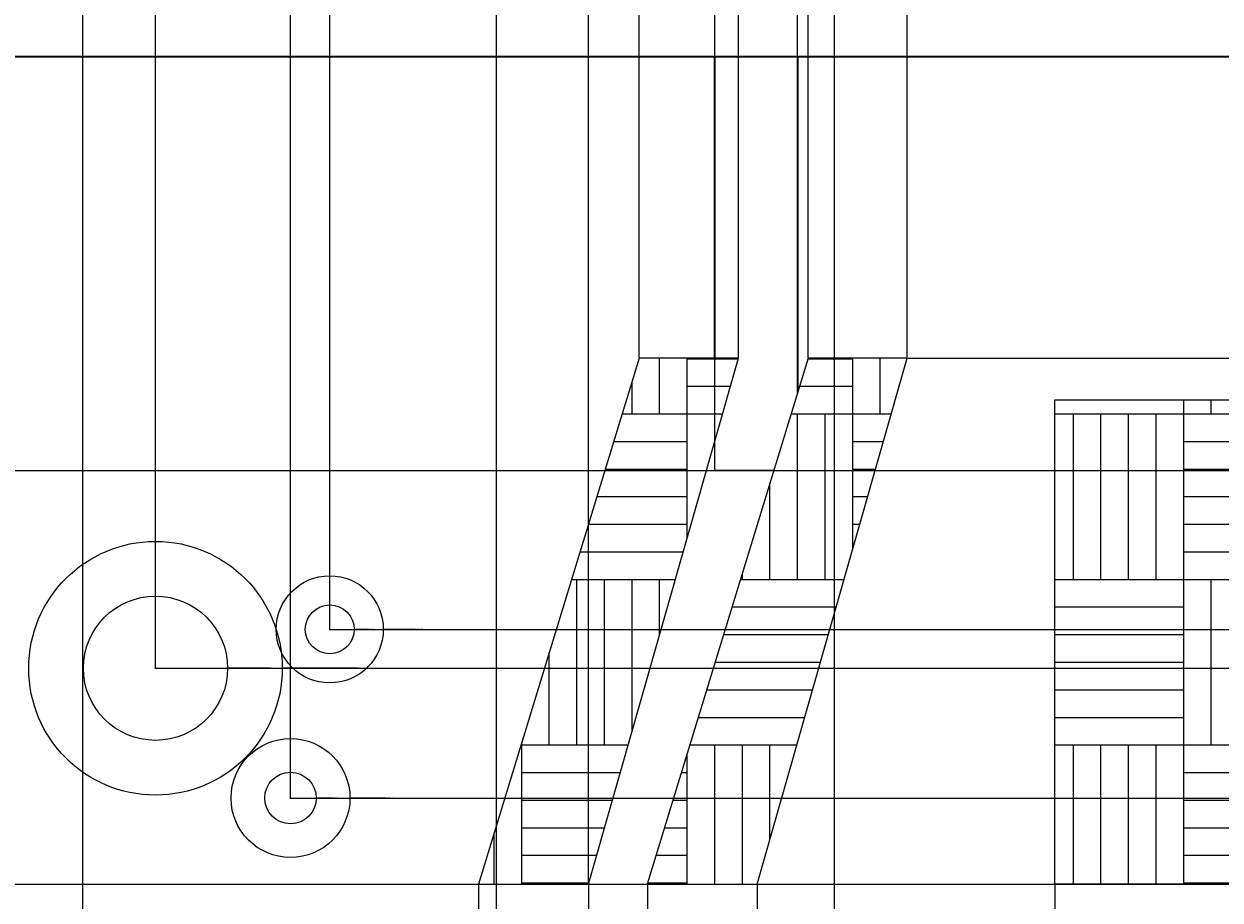
# Model space of a CAD drawing. Units: inches. Extents: x -15 to 605, y -220 to 570.
# Tile 4 of 10: x 265 to 438, y -118 to 9. Entities that reach past the tile are written whole.
import ezdxf

# ---------------------------------------------------------------- set-up
doc = ezdxf.new("R2010")
doc.units = ezdxf.units.IN
doc.header["$MEASUREMENT"] = 0
for name, color, linetype, lineweight in [('A-ANNO-DIMS', 2, 'Continuous', 18), ('A-COLS', 7, 'Continuous', 35), ('A-ELEV', 7, 'Continuous', 35), ('A-ELEV-PATT', 8, 'Continuous', 13), ('C-SITE', 3, 'Continuous', 25)]:
    doc.layers.add(name, color=color, linetype=linetype, lineweight=lineweight)
doc.styles.get("Standard").update_dxf_attribs({"font": 'arial.ttf'})
doc.dimstyles.get("Standard").update_dxf_attribs({"dimtxt": 0.18, "dimasz": 0.18, "dimexe": 0.18, "dimexo": 0.0625, "dimgap": 0.09, "dimtad": 0, "dimtih": 1, "dimtoh": 1, "dimdec": 4, "dimzin": 0, "dimdsep": 46, "dimtxsty": 'Standard', "dimcen": 0.09, "dimadec": 0, "dimazin": 0, "dimtfac": 1, "dimtdec": 4, "dimtofl": 0, "dimtmove": 0, "dimatfit": 3, "dimfxl": 1, "dimtolj": 1, "dimtzin": 0, "dimarcsym": 0})

# ---------------------------------------------------------------- blocks, each defined once
blk = doc.blocks.new('*D7')
at = {"layer": 'A-ANNO-DIMS', "color": 0, "lineweight": -2, "transparency": 16777216}
for p, q in [((23.99, 3.76), (23.99, -154.76)), ((566.72, -116.24), (566.72, -154.76)), ((24.17, -154.58), (294.96, -154.58)), ((566.54, -154.58), (295.75, -154.58))]:
    blk.add_line(p, q, dxfattribs=at)
at = {"layer": 'A-ANNO-DIMS', "color": 0, "transparency": 16777216}
for points in [[(24.17, -154.55), (24.17, -154.61), (23.99, -154.58)], [(566.54, -154.55), (566.54, -154.61), (566.72, -154.58)]]:
    blk.add_solid(points, dxfattribs=at)
at = {"layer": 'Defpoints', "color": 0, "transparency": 16777216}
for p in [(23.99, 3.82), (566.72, -116.18), (566.72, -154.58)]:
    blk.add_point(p, dxfattribs=at)
at = {"layer": 'A-ANNO-DIMS', "color": 0, "transparency": 16777216, "insert": (295.35, -154.58), "char_height": 0.18, "attachment_point": 5}
blk.add_mtext('\\A1;542.7', dxfattribs=at)
blk = doc.blocks.new('*D8')
at = {"layer": 'A-ANNO-DIMS', "color": 0, "lineweight": -2, "transparency": 16777216}
for p, q in [((23.99, 3.88), (23.99, 570.4)), ((24.17, 570.22), (263.7, 570.22)), ((503.81, 570.22), (264.28, 570.22)), ((503.99, 531.88), (503.99, 570.4))]:
    blk.add_line(p, q, dxfattribs=at)
at = {"layer": 'A-ANNO-DIMS', "color": 0, "transparency": 16777216}
for points in [[(24.17, 570.25), (24.17, 570.19), (23.99, 570.22)], [(503.81, 570.25), (503.81, 570.19), (503.99, 570.22)]]:
    blk.add_solid(points, dxfattribs=at)
at = {"layer": 'Defpoints', "color": 0, "transparency": 16777216}
for p in [(503.99, 570.22), (503.99, 531.82), (23.99, 3.82)]:
    blk.add_point(p, dxfattribs=at)
at = {"layer": 'A-ANNO-DIMS', "color": 0, "transparency": 16777216, "insert": (263.99, 570.22), "char_height": 0.18, "attachment_point": 5}
blk.add_mtext('\\A1;480', dxfattribs=at)
blk = doc.blocks.new('*D9')
at = {"layer": 'A-ANNO-DIMS', "color": 0, "lineweight": -2, "transparency": 16777216}
for p, q in [((503.92, 531.82), (-14.59, 531.82)), ((-14.41, 531.64), (-14.41, 208)), ((-14.41, -116), (-14.41, 207.64)), ((23.92, -116.18), (-14.59, -116.18))]:
    blk.add_line(p, q, dxfattribs=at)
at = {"layer": 'A-ANNO-DIMS', "color": 0, "transparency": 16777216}
for points in [[(-14.44, 531.64), (-14.38, 531.64), (-14.41, 531.82)], [(-14.44, -116), (-14.38, -116), (-14.41, -116.18)]]:
    blk.add_solid(points, dxfattribs=at)
at = {"layer": 'Defpoints', "color": 0, "transparency": 16777216}
for p in [(-14.41, 531.82), (503.99, 531.82), (23.99, -116.18)]:
    blk.add_point(p, dxfattribs=at)
at = {"layer": 'A-ANNO-DIMS', "color": 0, "transparency": 16777216, "insert": (-14.41, 207.82), "char_height": 0.18, "attachment_point": 5}
blk.add_mtext('\\A1;648', dxfattribs=at)
blk = doc.blocks.new('*D28')
at = {"layer": 'A-ANNO-DIMS', "color": 0, "lineweight": -2, "transparency": 16777216}
for p, q in [((260.99, 15.76), (260.99, -154.76)), ((272.99, 15.76), (272.99, -154.76)), ((261.17, -154.58), (266.78, -154.58)), ((272.81, -154.58), (267.2, -154.58))]:
    blk.add_line(p, q, dxfattribs=at)
at = {"layer": 'A-ANNO-DIMS', "color": 0, "transparency": 16777216}
for points in [[(261.17, -154.55), (261.17, -154.61), (260.99, -154.58)], [(272.81, -154.55), (272.81, -154.61), (272.99, -154.58)]]:
    blk.add_solid(points, dxfattribs=at)
at = {"layer": 'Defpoints', "color": 0, "transparency": 16777216}
for p in [(260.99, 15.82), (272.99, 15.82), (272.99, -154.58)]:
    blk.add_point(p, dxfattribs=at)
at = {"layer": 'A-ANNO-DIMS', "color": 0, "transparency": 16777216, "insert": (266.99, -154.58), "char_height": 0.18, "attachment_point": 5}
blk.add_mtext('\\A1;12', dxfattribs=at)
blk = doc.blocks.new('*D29')
at = {"layer": 'A-ANNO-DIMS', "color": 0, "lineweight": -2, "transparency": 16777216}
for p, q in [((272.99, 15.76), (272.99, -154.76)), ((332.99, 15.76), (332.99, -154.76)), ((273.17, -154.58), (302.77, -154.58)), ((332.81, -154.58), (303.21, -154.58))]:
    blk.add_line(p, q, dxfattribs=at)
at = {"layer": 'A-ANNO-DIMS', "color": 0, "transparency": 16777216}
for points in [[(273.17, -154.55), (273.17, -154.61), (272.99, -154.58)], [(332.81, -154.55), (332.81, -154.61), (332.99, -154.58)]]:
    blk.add_solid(points, dxfattribs=at)
at = {"layer": 'Defpoints', "color": 0, "transparency": 16777216}
for p in [(272.99, 15.82), (332.99, 15.82), (332.99, -154.58)]:
    blk.add_point(p, dxfattribs=at)
at = {"layer": 'A-ANNO-DIMS', "color": 0, "transparency": 16777216, "insert": (302.99, -154.58), "char_height": 0.18, "attachment_point": 5}
blk.add_mtext('\\A1;60', dxfattribs=at)
blk = doc.blocks.new('*D30')
at = {"layer": 'A-ANNO-DIMS', "color": 0, "lineweight": -2, "transparency": 16777216}
for p, q in [((382.03, 34.31), (382.03, -154.76)), ((332.99, 15.76), (332.99, -154.76)), ((333.17, -154.58), (357.11, -154.58)), ((381.85, -154.58), (357.91, -154.58))]:
    blk.add_line(p, q, dxfattribs=at)
at = {"layer": 'A-ANNO-DIMS', "color": 0, "transparency": 16777216}
for points in [[(333.17, -154.55), (333.17, -154.61), (332.99, -154.58)], [(381.85, -154.55), (381.85, -154.61), (382.03, -154.58)]]:
    blk.add_solid(points, dxfattribs=at)
at = {"layer": 'Defpoints', "color": 0, "transparency": 16777216}
for p in [(382.03, 34.38), (332.99, 15.82), (382.03, -154.58)]:
    blk.add_point(p, dxfattribs=at)
at = {"layer": 'A-ANNO-DIMS', "color": 0, "transparency": 16777216, "insert": (357.51, -154.58), "char_height": 0.18, "attachment_point": 5}
blk.add_mtext('\\A1;49.04', dxfattribs=at)
blk = doc.blocks.new('*D31')
at = {"layer": 'A-ANNO-DIMS', "color": 0, "lineweight": -2, "transparency": 16777216}
for p, q in [((382.03, 34.31), (382.03, -154.76)), ((491.99, 15.76), (491.99, -154.76)), ((382.21, -154.58), (436.55, -154.58)), ((491.81, -154.58), (437.46, -154.58))]:
    blk.add_line(p, q, dxfattribs=at)
at = {"layer": 'A-ANNO-DIMS', "color": 0, "transparency": 16777216}
for points in [[(382.21, -154.55), (382.21, -154.61), (382.03, -154.58)], [(491.81, -154.55), (491.81, -154.61), (491.99, -154.58)]]:
    blk.add_solid(points, dxfattribs=at)
at = {"layer": 'Defpoints', "color": 0, "transparency": 16777216}
for p in [(382.03, 34.38), (491.99, 15.82), (491.99, -154.58)]:
    blk.add_point(p, dxfattribs=at)
at = {"layer": 'A-ANNO-DIMS', "color": 0, "transparency": 16777216, "insert": (437.01, -154.58), "char_height": 0.18, "attachment_point": 5}
blk.add_mtext('\\A1;109.96', dxfattribs=at)
blk = doc.blocks.new('*D46')
at = {"layer": 'A-ANNO-DIMS', "color": 0, "lineweight": -2, "transparency": 16777216}
for p, q in [((251.99, -116.24), (251.99, -154.76)), ((330.43, -116.24), (330.43, -154.76)), ((252.17, -154.58), (290.82, -154.58)), ((330.25, -154.58), (291.6, -154.58))]:
    blk.add_line(p, q, dxfattribs=at)
at = {"layer": 'A-ANNO-DIMS', "color": 0, "transparency": 16777216}
for points in [[(252.17, -154.55), (252.17, -154.61), (251.99, -154.58)], [(330.25, -154.55), (330.25, -154.61), (330.43, -154.58)]]:
    blk.add_solid(points, dxfattribs=at)
at = {"layer": 'Defpoints', "color": 0, "transparency": 16777216}
for p in [(251.99, -116.18), (330.43, -116.18), (330.43, -154.58)]:
    blk.add_point(p, dxfattribs=at)
at = {"layer": 'A-ANNO-DIMS', "color": 0, "transparency": 16777216, "insert": (291.21, -154.58), "char_height": 0.18, "attachment_point": 5}
blk.add_mtext('\\A1;78.45', dxfattribs=at)
blk = doc.blocks.new('*D47')
at = {"layer": 'A-ANNO-DIMS', "color": 0, "lineweight": -2, "transparency": 16777216}
for p, q in [((330.43, -116.24), (330.43, -154.76)), ((346.37, -116.24), (346.37, -154.76)), ((330.61, -154.58), (337.94, -154.58)), ((346.19, -154.58), (338.85, -154.58))]:
    blk.add_line(p, q, dxfattribs=at)
at = {"layer": 'A-ANNO-DIMS', "color": 0, "transparency": 16777216}
for points in [[(330.61, -154.55), (330.61, -154.61), (330.43, -154.58)], [(346.19, -154.55), (346.19, -154.61), (346.37, -154.58)]]:
    blk.add_solid(points, dxfattribs=at)
at = {"layer": 'Defpoints', "color": 0, "transparency": 16777216}
for p in [(330.43, -116.18), (346.37, -116.18), (346.37, -154.58)]:
    blk.add_point(p, dxfattribs=at)
at = {"layer": 'A-ANNO-DIMS', "color": 0, "transparency": 16777216, "insert": (338.4, -154.58), "char_height": 0.18, "attachment_point": 5}
blk.add_mtext('\\A1;15.934', dxfattribs=at)
blk = doc.blocks.new('*D48')
at = {"layer": 'A-ANNO-DIMS', "color": 0, "lineweight": -2, "transparency": 16777216}
for p, q in [((346.37, -116.24), (346.37, -154.76)), ((354.92, -116.24), (354.92, -154.76)), ((346.55, -154.58), (350.32, -154.58)), ((354.74, -154.58), (350.97, -154.58))]:
    blk.add_line(p, q, dxfattribs=at)
at = {"layer": 'A-ANNO-DIMS', "color": 0, "transparency": 16777216}
for points in [[(346.55, -154.55), (346.55, -154.61), (346.37, -154.58)], [(354.74, -154.55), (354.74, -154.61), (354.92, -154.58)]]:
    blk.add_solid(points, dxfattribs=at)
at = {"layer": 'Defpoints', "color": 0, "transparency": 16777216}
for p in [(346.37, -116.18), (354.92, -116.18), (354.92, -154.58)]:
    blk.add_point(p, dxfattribs=at)
at = {"layer": 'A-ANNO-DIMS', "color": 0, "transparency": 16777216, "insert": (350.64, -154.58), "char_height": 0.18, "attachment_point": 5}
blk.add_mtext('\\A1;8.55', dxfattribs=at)
blk = doc.blocks.new('*D49')
at = {"layer": 'A-ANNO-DIMS', "color": 0, "lineweight": -2, "transparency": 16777216}
for p, q in [((354.92, -116.24), (354.92, -154.76)), ((370.85, -116.24), (370.85, -154.76)), ((355.1, -154.58), (362.43, -154.58)), ((370.67, -154.58), (363.34, -154.58))]:
    blk.add_line(p, q, dxfattribs=at)
at = {"layer": 'A-ANNO-DIMS', "color": 0, "transparency": 16777216}
for points in [[(355.1, -154.55), (355.1, -154.61), (354.92, -154.58)], [(370.67, -154.55), (370.67, -154.61), (370.85, -154.58)]]:
    blk.add_solid(points, dxfattribs=at)
at = {"layer": 'Defpoints', "color": 0, "transparency": 16777216}
for p in [(354.92, -116.18), (370.85, -116.18), (370.85, -154.58)]:
    blk.add_point(p, dxfattribs=at)
at = {"layer": 'A-ANNO-DIMS', "color": 0, "transparency": 16777216, "insert": (362.88, -154.58), "char_height": 0.18, "attachment_point": 5}
blk.add_mtext('\\A1;15.934', dxfattribs=at)
blk = doc.blocks.new('*D50')
at = {"layer": 'A-ANNO-DIMS', "color": 0, "lineweight": -2, "transparency": 16777216}
for p, q in [((370.85, -116.24), (370.85, -154.76)), ((414, -116.24), (414, -154.76)), ((371.03, -154.58), (392.03, -154.58)), ((413.82, -154.58), (392.82, -154.58))]:
    blk.add_line(p, q, dxfattribs=at)
at = {"layer": 'A-ANNO-DIMS', "color": 0, "transparency": 16777216}
for points in [[(371.03, -154.55), (371.03, -154.61), (370.85, -154.58)], [(413.82, -154.55), (413.82, -154.61), (414, -154.58)]]:
    blk.add_solid(points, dxfattribs=at)
at = {"layer": 'Defpoints', "color": 0, "transparency": 16777216}
for p in [(370.85, -116.18), (414, -116.18), (414, -154.58)]:
    blk.add_point(p, dxfattribs=at)
at = {"layer": 'A-ANNO-DIMS', "color": 0, "transparency": 16777216, "insert": (392.42, -154.58), "char_height": 0.18, "attachment_point": 5}
blk.add_mtext('\\A1;43.15', dxfattribs=at)
blk = doc.blocks.new('*D51')
at = {"layer": 'A-ANNO-DIMS', "color": 0, "lineweight": -2, "transparency": 16777216}
for p, q in [((414, -116.24), (414, -154.76)), ((566.72, -116.24), (566.72, -154.76)), ((414.18, -154.58), (489.9, -154.58)), ((566.54, -154.58), (490.81, -154.58))]:
    blk.add_line(p, q, dxfattribs=at)
at = {"layer": 'A-ANNO-DIMS', "color": 0, "transparency": 16777216}
for points in [[(414.18, -154.55), (414.18, -154.61), (414, -154.58)], [(566.54, -154.55), (566.54, -154.61), (566.72, -154.58)]]:
    blk.add_solid(points, dxfattribs=at)
at = {"layer": 'Defpoints', "color": 0, "transparency": 16777216}
for p in [(414, -116.18), (566.72, -116.18), (566.72, -154.58)]:
    blk.add_point(p, dxfattribs=at)
at = {"layer": 'A-ANNO-DIMS', "color": 0, "transparency": 16777216, "insert": (490.36, -154.58), "char_height": 0.18, "attachment_point": 5}
blk.add_mtext('\\A1;152.72', dxfattribs=at)
blk = doc.blocks.new('*D56')
at = {"layer": 'A-ANNO-DIMS', "color": 0, "lineweight": -2, "transparency": 16777216}
for p, q in [((233.14, -31.58), (233.14, 570.4)), ((233.32, 570.22), (298.47, 570.22)), ((364.53, 570.22), (299.38, 570.22)), ((364.71, -56.12), (364.71, 570.4))]:
    blk.add_line(p, q, dxfattribs=at)
at = {"layer": 'A-ANNO-DIMS', "color": 0, "transparency": 16777216}
for points in [[(233.32, 570.25), (233.32, 570.19), (233.14, 570.22)], [(364.53, 570.25), (364.53, 570.19), (364.71, 570.22)]]:
    blk.add_solid(points, dxfattribs=at)
at = {"layer": 'Defpoints', "color": 0, "transparency": 16777216}
for p in [(364.71, 570.22), (233.14, -31.64), (364.71, -56.18)]:
    blk.add_point(p, dxfattribs=at)
at = {"layer": 'A-ANNO-DIMS', "color": 0, "transparency": 16777216, "insert": (298.93, 570.22), "char_height": 0.18, "attachment_point": 5}
blk.add_mtext('\\A1;131.56', dxfattribs=at)
blk = doc.blocks.new('*D57')
at = {"layer": 'A-ANNO-DIMS', "color": 0, "lineweight": -2, "transparency": 16777216}
for p, q in [((364.71, -56.12), (364.71, 570.4)), ((364.89, 570.22), (370.5, 570.22)), ((376.53, 570.22), (370.92, 570.22)), ((376.71, -44.82), (376.71, 570.4))]:
    blk.add_line(p, q, dxfattribs=at)
at = {"layer": 'A-ANNO-DIMS', "color": 0, "transparency": 16777216}
for points in [[(364.89, 570.25), (364.89, 570.19), (364.71, 570.22)], [(376.53, 570.25), (376.53, 570.19), (376.71, 570.22)]]:
    blk.add_solid(points, dxfattribs=at)
at = {"layer": 'Defpoints', "color": 0, "transparency": 16777216}
for p in [(376.71, 570.22), (376.71, -44.88), (364.71, -56.18)]:
    blk.add_point(p, dxfattribs=at)
at = {"layer": 'A-ANNO-DIMS', "color": 0, "transparency": 16777216, "insert": (370.71, 570.22), "char_height": 0.18, "attachment_point": 5}
blk.add_mtext('\\A1;12', dxfattribs=at)
blk = doc.blocks.new('*D58')
at = {"layer": 'A-ANNO-DIMS', "color": 0, "lineweight": -2, "transparency": 16777216}
for p, q in [((376.71, -44.82), (376.71, 570.4)), ((376.89, 570.22), (419.58, 570.22)), ((462.92, 570.22), (420.23, 570.22)), ((463.1, -45.87), (463.1, 570.4))]:
    blk.add_line(p, q, dxfattribs=at)
at = {"layer": 'A-ANNO-DIMS', "color": 0, "transparency": 16777216}
for points in [[(376.89, 570.25), (376.89, 570.19), (376.71, 570.22)], [(462.92, 570.25), (462.92, 570.19), (463.1, 570.22)]]:
    blk.add_solid(points, dxfattribs=at)
at = {"layer": 'Defpoints', "color": 0, "transparency": 16777216}
for p in [(463.1, 570.22), (376.71, -44.88), (463.1, -45.94)]:
    blk.add_point(p, dxfattribs=at)
at = {"layer": 'A-ANNO-DIMS', "color": 0, "transparency": 16777216, "insert": (419.9, 570.22), "char_height": 0.18, "attachment_point": 5}
blk.add_mtext('\\A1;86.4', dxfattribs=at)
blk = doc.blocks.new('*D60')
at = {"layer": 'A-ANNO-DIMS', "color": 0, "lineweight": -2, "transparency": 16777216}
for p, q in [((346.37, -116.12), (346.37, 570.4)), ((346.55, 570.22), (349.67, 570.22)), ((353.57, 570.22), (350.45, 570.22)), ((353.75, -39.82), (353.75, 570.4))]:
    blk.add_line(p, q, dxfattribs=at)
at = {"layer": 'A-ANNO-DIMS', "color": 0, "transparency": 16777216}
for points in [[(346.55, 570.25), (346.55, 570.19), (346.37, 570.22)], [(353.57, 570.25), (353.57, 570.19), (353.75, 570.22)]]:
    blk.add_solid(points, dxfattribs=at)
at = {"layer": 'Defpoints', "color": 0, "transparency": 16777216}
for p in [(353.75, 570.22), (353.75, -39.88), (346.37, -116.18)]:
    blk.add_point(p, dxfattribs=at)
at = {"layer": 'A-ANNO-DIMS', "color": 0, "transparency": 16777216, "insert": (350.06, 570.22), "char_height": 0.18, "attachment_point": 5}
blk.add_mtext('\\A1;7.384', dxfattribs=at)
blk = doc.blocks.new('*D61')
at = {"layer": 'A-ANNO-DIMS', "color": 0, "lineweight": -2, "transparency": 16777216}
for p, q in [((353.75, -39.82), (353.75, 570.4)), ((353.93, 570.22), (360.55, 570.22)), ((367.95, 570.22), (361.33, 570.22)), ((368.13, -39.82), (368.13, 570.4))]:
    blk.add_line(p, q, dxfattribs=at)
at = {"layer": 'A-ANNO-DIMS', "color": 0, "transparency": 16777216}
for points in [[(353.93, 570.25), (353.93, 570.19), (353.75, 570.22)], [(367.95, 570.25), (367.95, 570.19), (368.13, 570.22)]]:
    blk.add_solid(points, dxfattribs=at)
at = {"layer": 'Defpoints', "color": 0, "transparency": 16777216}
for p in [(368.13, 570.22), (353.75, -39.88), (368.13, -39.88)]:
    blk.add_point(p, dxfattribs=at)
at = {"layer": 'A-ANNO-DIMS', "color": 0, "transparency": 16777216, "insert": (360.94, 570.22), "char_height": 0.18, "attachment_point": 5}
blk.add_mtext('\\A1;14.38', dxfattribs=at)
blk = doc.blocks.new('*D62')
at = {"layer": 'A-ANNO-DIMS', "color": 0, "lineweight": -2, "transparency": 16777216}
for p, q in [((378.23, -39.82), (378.23, 570.4)), ((378.41, 570.22), (385.04, 570.22)), ((392.43, 570.22), (385.81, 570.22)), ((392.61, -39.82), (392.61, 570.4))]:
    blk.add_line(p, q, dxfattribs=at)
at = {"layer": 'A-ANNO-DIMS', "color": 0, "transparency": 16777216}
for points in [[(378.41, 570.25), (378.41, 570.19), (378.23, 570.22)], [(392.43, 570.25), (392.43, 570.19), (392.61, 570.22)]]:
    blk.add_solid(points, dxfattribs=at)
at = {"layer": 'Defpoints', "color": 0, "transparency": 16777216}
for p in [(392.61, 570.22), (378.23, -39.88), (392.61, -39.88)]:
    blk.add_point(p, dxfattribs=at)
at = {"layer": 'A-ANNO-DIMS', "color": 0, "transparency": 16777216, "insert": (385.42, 570.22), "char_height": 0.18, "attachment_point": 5}
blk.add_mtext('\\A1;14.38', dxfattribs=at)
blk = doc.blocks.new('*D63')
at = {"layer": 'A-ANNO-DIMS', "color": 0, "lineweight": -2, "transparency": 16777216}
for p, q in [((392.68, -39.88), (605.3, -39.88)), ((605.12, -40.06), (605.12, -77.85)), ((605.12, -116), (605.12, -78.21)), ((370.91, -116.18), (605.3, -116.18))]:
    blk.add_line(p, q, dxfattribs=at)
at = {"layer": 'A-ANNO-DIMS', "color": 0, "transparency": 16777216}
for points in [[(605.09, -40.06), (605.15, -40.06), (605.12, -39.88)], [(605.09, -116), (605.15, -116), (605.12, -116.18)]]:
    blk.add_solid(points, dxfattribs=at)
at = {"layer": 'Defpoints', "color": 0, "transparency": 16777216}
for p in [(392.61, -39.88), (605.12, -39.88), (370.85, -116.18)]:
    blk.add_point(p, dxfattribs=at)
at = {"layer": 'A-ANNO-DIMS', "color": 0, "transparency": 16777216, "insert": (605.12, -78.03), "char_height": 0.18, "attachment_point": 5}
blk.add_mtext('\\A1;76.3', dxfattribs=at)
blk = doc.blocks.new('*D68')
at = {"layer": 'A-ANNO-DIMS', "color": 0, "lineweight": -2, "transparency": 16777216}
for p, q in [((252.05, -56.18), (605.3, -56.18)), ((605.12, -56.36), (605.12, -86)), ((605.12, -116), (605.12, -86.36)), ((252.05, -116.18), (605.3, -116.18))]:
    blk.add_line(p, q, dxfattribs=at)
at = {"layer": 'A-ANNO-DIMS', "color": 0, "transparency": 16777216}
for points in [[(605.09, -56.36), (605.15, -56.36), (605.12, -56.18)], [(605.09, -116), (605.15, -116), (605.12, -116.18)]]:
    blk.add_solid(points, dxfattribs=at)
at = {"layer": 'Defpoints', "color": 0, "transparency": 16777216}
for p in [(251.99, -56.18), (605.12, -56.18), (251.99, -116.18)]:
    blk.add_point(p, dxfattribs=at)
at = {"layer": 'A-ANNO-DIMS', "color": 0, "transparency": 16777216, "insert": (605.12, -86.18), "char_height": 0.18, "attachment_point": 5}
blk.add_mtext('\\A1;60', dxfattribs=at)
blk = doc.blocks.new('*D100')
at = {"layer": 'A-ANNO-DIMS', "color": 0, "lineweight": -2, "transparency": 16777216}
for p, q in [((283.5, -84.86), (283.68, -84.86)), ((283.59, -84.95), (283.59, -84.77)), ((313.01, -84.86), (302.16, -84.86))]:
    blk.add_line(p, q, dxfattribs=at)
at = {"layer": 'A-ANNO-DIMS', "color": 0, "transparency": 16777216}
blk.add_solid([(302.16, -84.83), (302.16, -84.89), (301.98, -84.86)], dxfattribs=at)
at = {"layer": 'Defpoints', "color": 0, "transparency": 16777216}
for p in [(265.2, -84.86), (301.98, -84.86)]:
    blk.add_point(p, dxfattribs=at)
at = {"layer": 'A-ANNO-DIMS', "color": 0, "transparency": 16777216, "insert": (313.5, -84.86), "char_height": 0.18, "attachment_point": 5}
blk.add_mtext('\\A1;∅36.78', dxfattribs=at)
blk = doc.blocks.new('*D101')
at = {"layer": 'A-ANNO-DIMS', "color": 0, "lineweight": -2, "transparency": 16777216}
for p, q in [((283.5, -84.86), (283.68, -84.86)), ((283.59, -84.95), (283.59, -84.77)), ((300.32, -84.86), (294.22, -84.86))]:
    blk.add_line(p, q, dxfattribs=at)
at = {"layer": 'A-ANNO-DIMS', "color": 0, "transparency": 16777216}
blk.add_solid([(294.22, -84.83), (294.22, -84.89), (294.04, -84.86)], dxfattribs=at)
at = {"layer": 'Defpoints', "color": 0, "transparency": 16777216}
for p in [(273.13, -84.86), (294.04, -84.86)]:
    blk.add_point(p, dxfattribs=at)
at = {"layer": 'A-ANNO-DIMS', "color": 0, "transparency": 16777216, "insert": (300.88, -84.86), "char_height": 0.18, "attachment_point": 5}
blk.add_mtext('\\A1;∅20.913', dxfattribs=at)
blk = doc.blocks.new('*D102')
at = {"layer": 'A-ANNO-DIMS', "color": 0, "lineweight": -2, "transparency": 16777216}
for p, q in [((303.08, -103.68), (303.26, -103.68)), ((303.17, -103.77), (303.17, -103.59)), ((316.97, -103.68), (311.97, -103.68))]:
    blk.add_line(p, q, dxfattribs=at)
at = {"layer": 'A-ANNO-DIMS', "color": 0, "transparency": 16777216}
blk.add_solid([(311.97, -103.65), (311.97, -103.71), (311.79, -103.68)], dxfattribs=at)
at = {"layer": 'Defpoints', "color": 0, "transparency": 16777216}
for p in [(294.55, -103.68), (311.79, -103.68)]:
    blk.add_point(p, dxfattribs=at)
at = {"layer": 'A-ANNO-DIMS', "color": 0, "transparency": 16777216, "insert": (317.53, -103.68), "char_height": 0.18, "attachment_point": 5}
blk.add_mtext('\\A1;∅17.243', dxfattribs=at)
blk = doc.blocks.new('*D103')
at = {"layer": 'A-ANNO-DIMS', "color": 0, "lineweight": -2, "transparency": 16777216}
for p, q in [((308.77, -79.22), (308.95, -79.22)), ((308.86, -79.31), (308.86, -79.13)), ((321.29, -79.22), (316.81, -79.22))]:
    blk.add_line(p, q, dxfattribs=at)
at = {"layer": 'A-ANNO-DIMS', "color": 0, "transparency": 16777216}
blk.add_solid([(316.81, -79.19), (316.81, -79.25), (316.63, -79.22)], dxfattribs=at)
at = {"layer": 'Defpoints', "color": 0, "transparency": 16777216}
for p in [(301.09, -79.22), (316.63, -79.22)]:
    blk.add_point(p, dxfattribs=at)
at = {"layer": 'A-ANNO-DIMS', "color": 0, "transparency": 16777216, "insert": (321.85, -79.22), "char_height": 0.18, "attachment_point": 5}
blk.add_mtext('\\A1;∅15.538', dxfattribs=at)
blk = doc.blocks.new('*D104')
at = {"layer": 'A-ANNO-DIMS', "color": 0, "lineweight": -2, "transparency": 16777216}
for p, q in [((251.99, -56.12), (251.99, 570.4)), ((252.17, 570.22), (267.39, 570.22)), ((283.41, 570.22), (268.18, 570.22)), ((283.59, -84.79), (283.59, 570.4))]:
    blk.add_line(p, q, dxfattribs=at)
at = {"layer": 'A-ANNO-DIMS', "color": 0, "transparency": 16777216}
for points in [[(252.17, 570.25), (252.17, 570.19), (251.99, 570.22)], [(283.41, 570.25), (283.41, 570.19), (283.59, 570.22)]]:
    blk.add_solid(points, dxfattribs=at)
at = {"layer": 'Defpoints', "color": 0, "transparency": 16777216}
for p in [(283.59, 570.22), (251.99, -56.18), (283.59, -84.86)]:
    blk.add_point(p, dxfattribs=at)
at = {"layer": 'A-ANNO-DIMS', "color": 0, "transparency": 16777216, "insert": (267.79, 570.22), "char_height": 0.18, "attachment_point": 5}
blk.add_mtext('\\A1;31.60', dxfattribs=at)
blk = doc.blocks.new('*D105')
at = {"layer": 'A-ANNO-DIMS', "color": 0, "lineweight": -2, "transparency": 16777216}
for p, q in [((283.59, -84.79), (283.59, 570.4)), ((283.77, 570.22), (292.92, 570.22)), ((302.99, 570.22), (293.84, 570.22)), ((303.17, -103.62), (303.17, 570.4))]:
    blk.add_line(p, q, dxfattribs=at)
at = {"layer": 'A-ANNO-DIMS', "color": 0, "transparency": 16777216}
for points in [[(283.77, 570.25), (283.77, 570.19), (283.59, 570.22)], [(302.99, 570.25), (302.99, 570.19), (303.17, 570.22)]]:
    blk.add_solid(points, dxfattribs=at)
at = {"layer": 'Defpoints', "color": 0, "transparency": 16777216}
for p in [(303.17, 570.22), (283.59, -84.86), (303.17, -103.68)]:
    blk.add_point(p, dxfattribs=at)
at = {"layer": 'A-ANNO-DIMS', "color": 0, "transparency": 16777216, "insert": (293.38, 570.22), "char_height": 0.18, "attachment_point": 5}
blk.add_mtext('\\A1;19.585', dxfattribs=at)
blk = doc.blocks.new('*D106')
at = {"layer": 'A-ANNO-DIMS', "color": 0, "lineweight": -2, "transparency": 16777216}
for p, q in [((303.17, -103.62), (303.17, 570.4)), ((303.35, 570.22), (305.62, 570.22)), ((308.68, 570.22), (306.41, 570.22)), ((308.86, -79.16), (308.86, 570.4))]:
    blk.add_line(p, q, dxfattribs=at)
at = {"layer": 'A-ANNO-DIMS', "color": 0, "transparency": 16777216}
for points in [[(303.35, 570.25), (303.35, 570.19), (303.17, 570.22)], [(308.68, 570.25), (308.68, 570.19), (308.86, 570.22)]]:
    blk.add_solid(points, dxfattribs=at)
at = {"layer": 'Defpoints', "color": 0, "transparency": 16777216}
for p in [(308.86, 570.22), (308.86, -79.22), (303.17, -103.68)]:
    blk.add_point(p, dxfattribs=at)
at = {"layer": 'A-ANNO-DIMS', "color": 0, "transparency": 16777216, "insert": (306.02, 570.22), "char_height": 0.18, "attachment_point": 5}
blk.add_mtext('\\A1;5.689', dxfattribs=at)
blk = doc.blocks.new('*D107')
at = {"layer": 'A-ANNO-DIMS', "color": 0, "lineweight": -2, "transparency": 16777216}
for p, q in [((303.23, -103.68), (605.3, -103.68)), ((605.12, -103.86), (605.12, -109.75)), ((605.12, -116), (605.12, -110.11)), ((330.5, -116.18), (605.3, -116.18))]:
    blk.add_line(p, q, dxfattribs=at)
at = {"layer": 'A-ANNO-DIMS', "color": 0, "transparency": 16777216}
for points in [[(605.09, -103.86), (605.15, -103.86), (605.12, -103.68)], [(605.09, -116), (605.15, -116), (605.12, -116.18)]]:
    blk.add_solid(points, dxfattribs=at)
at = {"layer": 'Defpoints', "color": 0, "transparency": 16777216}
for p in [(303.17, -103.68), (605.12, -103.68), (330.43, -116.18)]:
    blk.add_point(p, dxfattribs=at)
at = {"layer": 'A-ANNO-DIMS', "color": 0, "transparency": 16777216, "insert": (605.12, -109.93), "char_height": 0.18, "attachment_point": 5}
blk.add_mtext('\\A1;12.503', dxfattribs=at)
blk = doc.blocks.new('*D108')
at = {"layer": 'A-ANNO-DIMS', "color": 0, "lineweight": -2, "transparency": 16777216}
for p, q in [((283.65, -84.86), (605.3, -84.86)), ((605.12, -85.04), (605.12, -94.09)), ((605.12, -103.5), (605.12, -94.45)), ((303.23, -103.68), (605.3, -103.68))]:
    blk.add_line(p, q, dxfattribs=at)
at = {"layer": 'A-ANNO-DIMS', "color": 0, "transparency": 16777216}
for points in [[(605.09, -85.04), (605.15, -85.04), (605.12, -84.86)], [(605.09, -103.5), (605.15, -103.5), (605.12, -103.68)]]:
    blk.add_solid(points, dxfattribs=at)
at = {"layer": 'Defpoints', "color": 0, "transparency": 16777216}
for p in [(283.59, -84.86), (605.12, -84.86), (303.17, -103.68)]:
    blk.add_point(p, dxfattribs=at)
at = {"layer": 'A-ANNO-DIMS', "color": 0, "transparency": 16777216, "insert": (605.12, -94.27), "char_height": 0.18, "attachment_point": 5}
blk.add_mtext('\\A1;18.82', dxfattribs=at)
blk = doc.blocks.new('*D109')
at = {"layer": 'A-ANNO-DIMS', "color": 0, "lineweight": -2, "transparency": 16777216}
for p, q in [((308.92, -79.22), (605.3, -79.22)), ((605.12, -79.4), (605.12, -81.86)), ((605.12, -84.68), (605.12, -82.22)), ((283.65, -84.86), (605.3, -84.86))]:
    blk.add_line(p, q, dxfattribs=at)
at = {"layer": 'A-ANNO-DIMS', "color": 0, "transparency": 16777216}
for points in [[(605.09, -79.4), (605.15, -79.4), (605.12, -79.22)], [(605.09, -84.68), (605.15, -84.68), (605.12, -84.86)]]:
    blk.add_solid(points, dxfattribs=at)
at = {"layer": 'Defpoints', "color": 0, "transparency": 16777216}
for p in [(308.86, -79.22), (605.12, -79.22), (283.59, -84.86)]:
    blk.add_point(p, dxfattribs=at)
at = {"layer": 'A-ANNO-DIMS', "color": 0, "transparency": 16777216, "insert": (605.12, -82.04), "char_height": 0.18, "attachment_point": 5}
blk.add_mtext('\\A1;5.637', dxfattribs=at)
blk = doc.blocks.new('*D115')
at = {"layer": 'A-ANNO-DIMS', "color": 0, "lineweight": -2, "transparency": 16777216}
for p, q in [((283.5, -84.86), (283.68, -84.86)), ((283.59, -84.95), (283.59, -84.77)), ((313.01, -84.86), (302.16, -84.86))]:
    blk.add_line(p, q, dxfattribs=at)
at = {"layer": 'A-ANNO-DIMS', "color": 0, "transparency": 16777216}
blk.add_solid([(302.16, -84.83), (302.16, -84.89), (301.98, -84.86)], dxfattribs=at)
at = {"layer": 'Defpoints', "color": 0, "transparency": 16777216}
for p in [(265.2, -84.85), (301.98, -84.86)]:
    blk.add_point(p, dxfattribs=at)
at = {"layer": 'A-ANNO-DIMS', "color": 0, "transparency": 16777216, "insert": (313.5, -84.86), "char_height": 0.18, "attachment_point": 5}
blk.add_mtext('\\A1;∅36.78', dxfattribs=at)
blk = doc.blocks.new('*D116')
at = {"layer": 'A-ANNO-DIMS', "color": 0, "lineweight": -2, "transparency": 16777216}
for p, q in [((283.5, -84.86), (283.68, -84.86)), ((283.59, -84.95), (283.59, -84.77)), ((300.32, -84.86), (294.22, -84.86))]:
    blk.add_line(p, q, dxfattribs=at)
at = {"layer": 'A-ANNO-DIMS', "color": 0, "transparency": 16777216}
blk.add_solid([(294.22, -84.83), (294.22, -84.89), (294.04, -84.86)], dxfattribs=at)
at = {"layer": 'Defpoints', "color": 0, "transparency": 16777216}
for p in [(273.13, -84.85), (294.04, -84.86)]:
    blk.add_point(p, dxfattribs=at)
at = {"layer": 'A-ANNO-DIMS', "color": 0, "transparency": 16777216, "insert": (300.88, -84.86), "char_height": 0.18, "attachment_point": 5}
blk.add_mtext('\\A1;∅20.913', dxfattribs=at)
blk = doc.blocks.new('*D117')
at = {"layer": 'A-ANNO-DIMS', "color": 0, "lineweight": -2, "transparency": 16777216}
for p, q in [((308.77, -79.22), (308.95, -79.22)), ((308.86, -79.31), (308.86, -79.13)), ((321.29, -79.22), (316.81, -79.22))]:
    blk.add_line(p, q, dxfattribs=at)
at = {"layer": 'A-ANNO-DIMS', "color": 0, "transparency": 16777216}
blk.add_solid([(316.81, -79.19), (316.81, -79.25), (316.63, -79.22)], dxfattribs=at)
at = {"layer": 'Defpoints', "color": 0, "transparency": 16777216}
for p in [(301.09, -79.22), (316.63, -79.22)]:
    blk.add_point(p, dxfattribs=at)
at = {"layer": 'A-ANNO-DIMS', "color": 0, "transparency": 16777216, "insert": (321.85, -79.22), "char_height": 0.18, "attachment_point": 5}
blk.add_mtext('\\A1;∅15.538', dxfattribs=at)
blk = doc.blocks.new('*D118')
at = {"layer": 'A-ANNO-DIMS', "color": 0, "lineweight": -2, "transparency": 16777216}
for p, q in [((308.77, -79.22), (308.95, -79.22)), ((308.86, -79.31), (308.86, -79.13)), ((314.53, -79.22), (312.59, -79.22))]:
    blk.add_line(p, q, dxfattribs=at)
at = {"layer": 'A-ANNO-DIMS', "color": 0, "transparency": 16777216}
blk.add_solid([(312.59, -79.19), (312.59, -79.25), (312.41, -79.22)], dxfattribs=at)
at = {"layer": 'Defpoints', "color": 0, "transparency": 16777216}
for p in [(305.32, -79.22), (312.41, -79.22)]:
    blk.add_point(p, dxfattribs=at)
at = {"layer": 'A-ANNO-DIMS', "color": 0, "transparency": 16777216, "insert": (315.01, -79.22), "char_height": 0.18, "attachment_point": 5}
blk.add_mtext('\\A1;∅7.091', dxfattribs=at)
blk = doc.blocks.new('*D119')
at = {"layer": 'A-ANNO-DIMS', "color": 0, "lineweight": -2, "transparency": 16777216}
for p, q in [((303.08, -103.68), (303.26, -103.68)), ((303.17, -103.77), (303.17, -103.59)), ((316.97, -103.68), (311.97, -103.68))]:
    blk.add_line(p, q, dxfattribs=at)
at = {"layer": 'A-ANNO-DIMS', "color": 0, "transparency": 16777216}
blk.add_solid([(311.97, -103.65), (311.97, -103.71), (311.79, -103.68)], dxfattribs=at)
at = {"layer": 'Defpoints', "color": 0, "transparency": 16777216}
for p in [(294.55, -103.68), (311.79, -103.68)]:
    blk.add_point(p, dxfattribs=at)
at = {"layer": 'A-ANNO-DIMS', "color": 0, "transparency": 16777216, "insert": (317.53, -103.68), "char_height": 0.18, "attachment_point": 5}
blk.add_mtext('\\A1;∅17.243', dxfattribs=at)
blk = doc.blocks.new('*D120')
at = {"layer": 'A-ANNO-DIMS', "color": 0, "lineweight": -2, "transparency": 16777216}
for p, q in [((303.08, -103.68), (303.26, -103.68)), ((303.17, -103.77), (303.17, -103.59)), ((309.15, -103.68), (307.09, -103.68))]:
    blk.add_line(p, q, dxfattribs=at)
at = {"layer": 'A-ANNO-DIMS', "color": 0, "transparency": 16777216}
blk.add_solid([(307.09, -103.65), (307.09, -103.71), (306.91, -103.68)], dxfattribs=at)
at = {"layer": 'Defpoints', "color": 0, "transparency": 16777216}
for p in [(299.44, -103.68), (306.91, -103.68)]:
    blk.add_point(p, dxfattribs=at)
at = {"layer": 'A-ANNO-DIMS', "color": 0, "transparency": 16777216, "insert": (309.64, -103.68), "char_height": 0.18, "attachment_point": 5}
blk.add_mtext('\\A1;∅7.469', dxfattribs=at)

msp = doc.modelspace()

# ---------------------------------------------------------------- hatches: boundary and pattern name
at = {"layer": 'A-ELEV-PATT'}
h = msp.add_hatch(dxfattribs=at)
h.set_pattern_fill('AR-PARQ1', color=256, scale=2)
h.set_pattern_definition([(90, (-191.319, 0), (-24, 24), [24, -24]), (90, (-187.319, 0), (-24, 24), [24, -24]), (90, (-183.319, 0), (-24, 24), [24, -24]), (90, (-179.319, 0), (-24, 24), [24, -24]), (90, (-175.319, 0), (-24, 24), [24, -24]), (90, (-171.319, 0), (-24, 24), [24, -24]), (90, (-167.319, 0), (-24, 24), [24, -24]), (0, (-191.319, 24), (24, -24), [24, -24]), (0, (-191.319, 28), (24, -24), [24, -24]), (0, (-191.319, 32), (24, -24), [24, -24]), (0, (-191.319, 36), (24, -24), [24, -24]), (0, (-191.319, 40), (24, -24), [24, -24]), (0, (-191.319, 44), (24, -24), [24, -24]), (0, (-191.319, 48), (24, -24), [24, -24])])
h.paths.add_polyline_path([(392.6125, -39.8843), (378.2334, -39.8843), (354.916, -116.1813), (370.8496, -116.1813)])
h.paths.add_polyline_path([(368.1292, -39.8843), (353.7501, -39.8843), (330.4327, -116.1813), (346.3663, -116.1813)])
h.paths.add_polyline_path([(566.7161, -45.9373), (413.9976, -45.9373), (413.9976, -116.1813), (566.7161, -116.1813)])
h.paths.add_polyline_path([(251.9872, -35.1813), (227.9872, -35.1813), (227.9872, -116.1813), (251.9872, -116.1813)])
h.paths.add_polyline_path([(83.9872, -35.1813), (23.9872, -35.1813), (23.9872, -116.1813), (83.9872, -116.1813), (83.9872, -113.1422)])
h.paths.add_polyline_path([(72.6838, -44.8238), (72.6838, -109.4483), (32.7886, -109.4483), (32.7886, -44.8238)], flags=16)

# ---------------------------------------------------------------- linework, layer by layer
at = {"layer": 'A-COLS'}
msp.add_lwpolyline([(364.7066, -39.8843), (364.7066, 3.8187), (376.7066, 3.8187), (376.7066, -44.8803)], dxfattribs=at)
at = {"layer": 'A-ELEV'}
msp.add_lwpolyline([(23.9872, 123.8187), (23.9872, 3.8187), (503.9872, 3.8187), (503.9872, 123.8187), (503.9872, 531.8187)], dxfattribs=at)
at = {"layer": 'C-SITE'}
for p, q in [((251.9872, -56.1813), (348.7695, -56.1813)), ((363.4807, -56.1813), (373.2529, -56.1813)), ((387.964, -56.1813), (413.9976, -56.1813)), ((23.9872, -116.1813), (503.9872, -116.1813))]:
    msp.add_line(p, q, dxfattribs=at)
for points in [[(330.4327, -116.1813), (346.3663, -116.1813), (368.1292, -39.8843), (353.7501, -39.8843)], [(354.916, -116.1813), (370.8496, -116.1813), (392.6125, -39.8843), (378.2334, -39.8843)], [(413.9976, -45.9373), (566.7161, -45.9373), (566.7161, -116.1813), (413.9976, -116.1813)]]:
    msp.add_lwpolyline(points, close=True, dxfattribs=at)
msp.add_lwpolyline([(373.2529, -56.1813), (364.7066, -56.1813), (364.7066, -51.8834)], dxfattribs=at)
for centre, radius in [((283.5871, -84.8572), 18.3903), ((308.8611, -79.2202), 7.7688), ((283.5871, -84.8572), 10.4564), ((308.8611, -79.2202), 3.5457), ((303.1719, -103.6786), 8.6213), ((303.1719, -103.6786), 3.7344)]:
    msp.add_circle(centre, radius, dxfattribs=at)

# ---------------------------------------------------------------- dimensions: what is measured, and where the dimension line sits
at = {"layer": 'A-ANNO-DIMS'}
for base, p1, p2, override, picture, middle in [((503.9872, 570.2187), (23.9872, 3.8187), (503.9872, 531.8187), {"dimdec": 0, "dimlfac": 1, "dimrnd": 0, "dimzin": 0, "dimdsep": 46, "dimlunit": 2}, '*D8', (263.9872, 570.2187)), ((364.7066, 570.2187), (233.1439, -31.6396), (364.7066, -56.1813), {"dimdec": 2, "dimlfac": 1, "dimrnd": 0, "dimzin": 0, "dimdsep": 46, "dimlunit": 2}, '*D56', (298.9252, 570.2187)), ((283.5871, 570.2187), (251.9872, -56.1813), (283.5871, -84.8572), {"dimdec": 2, "dimlfac": 1, "dimrnd": 0, "dimzin": 0, "dimdsep": 46, "dimlunit": 2}, '*D104', (267.7872, 570.2187)), ((303.1719, 570.2187), (283.5871, -84.8572), (303.1719, -103.6786), {"dimdec": 3, "dimlfac": 1, "dimrnd": 0, "dimzin": 0, "dimdsep": 46, "dimlunit": 2}, '*D105', (293.3795, 570.2187)), ((308.8611, 570.2187), (303.1719, -103.6786), (308.8611, -79.2202), {"dimdec": 3, "dimlfac": 1, "dimrnd": 0, "dimzin": 0, "dimdsep": 46, "dimlunit": 2}, '*D106', (306.0165, 570.2187)), ((353.7501, 570.2187), (346.3663, -116.1813), (353.7501, -39.8843), {"dimdec": 3, "dimlfac": 1, "dimrnd": 0, "dimzin": 0, "dimdsep": 46, "dimlunit": 2}, '*D60', (350.0582, 570.2187)), ((368.1292, 570.2187), (353.7501, -39.8843), (368.1292, -39.8843), {"dimdec": 2, "dimlfac": 1, "dimrnd": 0, "dimzin": 0, "dimdsep": 46, "dimlunit": 2}, '*D61', (360.9397, 570.2187)), ((376.7066, 570.2187), (364.7066, -56.1813), (376.7066, -44.8803), {"dimdec": 0, "dimlfac": 1, "dimrnd": 0, "dimzin": 0, "dimdsep": 46, "dimlunit": 2}, '*D57', (370.7066, 570.2187)), ((463.1032, 570.2187), (376.7066, -44.8803), (463.1032, -45.9373), {"dimdec": 1, "dimlfac": 1, "dimrnd": 0, "dimzin": 0, "dimdsep": 46, "dimlunit": 2}, '*D58', (419.9049, 570.2187)), ((392.6125, 570.2187), (378.2334, -39.8843), (392.6125, -39.8843), {"dimdec": 2, "dimlfac": 1, "dimrnd": 0, "dimzin": 0, "dimdsep": 46, "dimlunit": 2}, '*D62', (385.423, 570.2187)), ((382.0304, -154.5813), (332.9872, 15.8187), (382.0304, 34.3758), {"dimdec": 2, "dimlfac": 1, "dimrnd": 0, "dimzin": 0, "dimdsep": 46, "dimlunit": 2}, '*D30', (357.5088, -154.5813)), ((491.9872, -154.5813), (382.0304, 34.3758), (491.9872, 15.8187), {"dimdec": 2, "dimlfac": 1, "dimrnd": 0, "dimzin": 0, "dimdsep": 46, "dimlunit": 2}, '*D31', (437.0088, -154.5813)), ((272.9872, -154.5813), (260.9872, 15.8187), (272.9872, 15.8187), {"dimdec": 0, "dimlfac": 1, "dimrnd": 0, "dimzin": 0, "dimdsep": 46, "dimlunit": 2}, '*D28', (266.9872, -154.5813)), ((332.9872, -154.5813), (272.9872, 15.8187), (332.9872, 15.8187), {"dimdec": 0, "dimlfac": 1, "dimrnd": 0, "dimzin": 0, "dimdsep": 46, "dimlunit": 2}, '*D29', (302.9872, -154.5813)), ((566.7161, -154.5813), (23.9872, 3.8187), (566.7161, -116.1813), {"dimdec": 1, "dimlfac": 1, "dimrnd": 0, "dimzin": 0, "dimdsep": 46, "dimlunit": 2}, '*D7', (295.3517, -154.5813)), ((330.4327, -154.5813), (251.9872, -116.1813), (330.4327, -116.1813), {"dimdec": 2, "dimlfac": 1, "dimrnd": 0, "dimzin": 0, "dimdsep": 46, "dimlunit": 2}, '*D46', (291.21, -154.5813)), ((346.3663, -154.5813), (330.4327, -116.1813), (346.3663, -116.1813), {"dimdec": 3, "dimlfac": 1, "dimrnd": 0, "dimzin": 0, "dimdsep": 46, "dimlunit": 2}, '*D47', (338.3995, -154.5813)), ((354.916, -154.5813), (346.3663, -116.1813), (354.916, -116.1813), {"dimdec": 2, "dimlfac": 1, "dimrnd": 0, "dimzin": 0, "dimdsep": 46, "dimlunit": 2}, '*D48', (350.6411, -154.5813)), ((370.8496, -154.5813), (354.916, -116.1813), (370.8496, -116.1813), {"dimdec": 3, "dimlfac": 1, "dimrnd": 0, "dimzin": 0, "dimdsep": 46, "dimlunit": 2}, '*D49', (362.8828, -154.5813)), ((413.9976, -154.5813), (370.8496, -116.1813), (413.9976, -116.1813), {"dimdec": 2, "dimlfac": 1, "dimrnd": 0, "dimzin": 0, "dimdsep": 46, "dimlunit": 2}, '*D50', (392.4236, -154.5813)), ((566.7161, -154.5813), (413.9976, -116.1813), (566.7161, -116.1813), {"dimdec": 2, "dimlfac": 1, "dimrnd": 0, "dimzin": 0, "dimdsep": 46, "dimlunit": 2}, '*D51', (490.3568, -154.5813))]:
    dim = msp.add_linear_dim(base=base, p1=p1, p2=p2, dimstyle='Standard', override=override, dxfattribs=at)
    dim.commit()
    dim.dimension.update_dxf_attribs({"geometry": picture, "text_midpoint": middle})
for base, p1, p2, override, picture, middle in [((-14.4128, 531.8187), (23.9872, -116.1813), (503.9872, 531.8187), {"dimdec": 0, "dimlfac": 1, "dimrnd": 0, "dimzin": 0, "dimdsep": 46, "dimlunit": 2}, '*D9', (-14.4128, 207.8187)), ((605.1161, -39.8843), (370.8496, -116.1813), (392.6125, -39.8843), {"dimdec": 1, "dimlfac": 1, "dimrnd": 0, "dimzin": 0, "dimdsep": 46, "dimlunit": 2}, '*D63', (605.1161, -78.0328)), ((605.1161, -56.1813), (251.9872, -116.1813), (251.9872, -56.1813), {"dimdec": 0, "dimlfac": 1, "dimrnd": 0, "dimzin": 0, "dimdsep": 46, "dimlunit": 2}, '*D68', (605.1161, -86.1813)), ((605.1161, -79.2202), (283.5871, -84.8572), (308.8611, -79.2202), {"dimdec": 3, "dimlfac": 1, "dimrnd": 0, "dimzin": 0, "dimdsep": 46, "dimlunit": 2}, '*D109', (605.1161, -82.0387)), ((605.1161, -84.8572), (303.1719, -103.6786), (283.5871, -84.8572), {"dimdec": 2, "dimlfac": 1, "dimrnd": 0, "dimzin": 0, "dimdsep": 46, "dimlunit": 2}, '*D108', (605.1161, -94.2679)), ((605.1161, -103.6786), (330.4327, -116.1813), (303.1719, -103.6786), {"dimdec": 3, "dimlfac": 1, "dimrnd": 0, "dimzin": 0, "dimdsep": 46, "dimlunit": 2}, '*D107', (605.1161, -109.9299))]:
    dim = msp.add_linear_dim(base=base, p1=p1, p2=p2, angle=90, dimstyle='Standard', override=override, dxfattribs=at)
    dim.commit()
    dim.dimension.update_dxf_attribs({"geometry": picture, "text_midpoint": middle})
for p1, p2, override, picture, middle in [((301.0923, -79.2205), (316.63, -79.22), {"dimdec": 3, "dimlfac": 1, "dimrnd": 0, "dimzin": 0, "dimdsep": 46, "dimlunit": 2}, '*D103', (321.2913, -79.2199)), ((301.0923, -79.2205), (316.63, -79.22), {"dimdec": 3, "dimlfac": 1, "dimrnd": 0, "dimzin": 0, "dimdsep": 46, "dimlunit": 2}, '*D117', (321.2913, -79.2199)), ((305.3155, -79.2205), (312.4068, -79.22), {"dimdec": 3, "dimlfac": 1, "dimrnd": 0, "dimzin": 0, "dimdsep": 46, "dimlunit": 2}, '*D118', (314.5342, -79.2199)), ((265.1968, -84.8573), (301.9775, -84.857), {"dimdec": 2, "dimlfac": 1, "dimrnd": 0, "dimzin": 0, "dimdsep": 46, "dimlunit": 2}, '*D100', (313.0117, -84.8569)), ((265.1968, -84.8543), (301.9775, -84.86), {"dimdec": 2, "dimlfac": 1, "dimrnd": 0, "dimzin": 0, "dimdsep": 46, "dimlunit": 2}, '*D115', (313.0117, -84.8617)), ((273.1308, -84.8573), (294.0435, -84.857), {"dimdec": 3, "dimlfac": 1, "dimrnd": 0, "dimzin": 0, "dimdsep": 46, "dimlunit": 2}, '*D101', (300.3173, -84.8569)), ((273.1308, -84.8543), (294.0435, -84.86), {"dimdec": 3, "dimlfac": 1, "dimrnd": 0, "dimzin": 0, "dimdsep": 46, "dimlunit": 2}, '*D116', (300.3173, -84.8617)), ((294.5506, -103.6782), (311.7932, -103.679), {"dimdec": 3, "dimlfac": 1, "dimrnd": 0, "dimzin": 0, "dimdsep": 46, "dimlunit": 2}, '*D102', (316.9659, -103.6792)), ((294.5506, -103.6772), (311.7932, -103.68), {"dimdec": 3, "dimlfac": 1, "dimrnd": 0, "dimzin": 0, "dimdsep": 46, "dimlunit": 2}, '*D119', (316.9659, -103.6808)), ((299.4375, -103.6772), (306.9063, -103.68), {"dimdec": 3, "dimlfac": 1, "dimrnd": 0, "dimzin": 0, "dimdsep": 46, "dimlunit": 2}, '*D120', (309.147, -103.6808))]:
    dim = msp.add_diameter_dim_2p(p1=p1, p2=p2, dimstyle='Standard', override=override, dxfattribs=at)
    dim.commit()
    dim.dimension.update_dxf_attribs({"geometry": picture, "text_midpoint": middle, "dimtype": 163})

doc.saveas('drawing.dxf')
